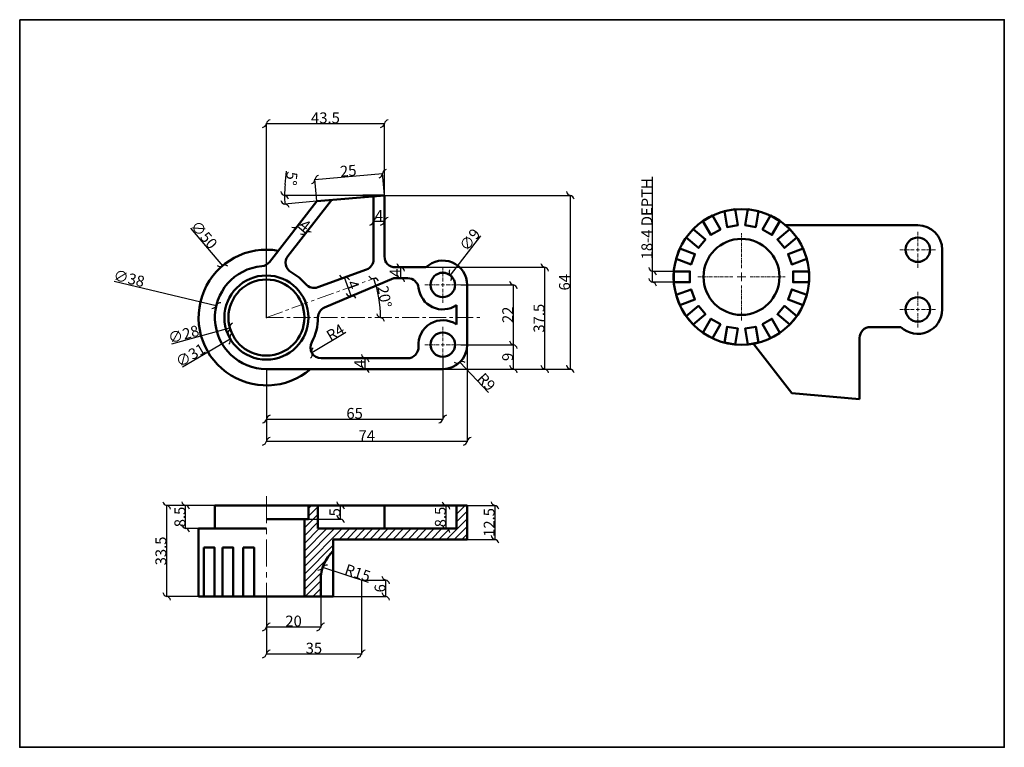
# Model space of a CAD drawing. Units: millimetres. Extents: x 359 to 722, y 83 to 351.
import ezdxf

# ---------------------------------------------------------------- set-up
doc = ezdxf.new("R2010")
doc.units = ezdxf.units.MM
doc.header["$MEASUREMENT"] = 0
doc.linetypes.add('CENTER', pattern=[2, 1.25, -0.25, 0.25, -0.25])
for name, color, linetype, lineweight in [('M-CNTR', 1, 'CENTER', 18), ('M-DIMS', 2, 'Continuous', 25), ('M-HATC', 8, 'Continuous', 18), ('M-OUTL', 7, 'Continuous', 50), ('M-TTLB', 7, 'Continuous', 35)]:
    doc.layers.add(name, color=color, linetype=linetype, lineweight=lineweight)
doc.styles.get("Standard").update_dxf_attribs({"font": 'arial.ttf'})
doc.dimstyles.get("Standard").update_dxf_attribs({"dimtxt": 4, "dimasz": 4, "dimexe": 0.18, "dimexo": 0.0625, "dimgap": 0.09, "dimtad": 1, "dimdec": 0, "dimzin": 0, "dimdsep": 46, "dimtxsty": 'Standard', "dimblk": 'INTEGRAL', "dimcen": 0.09, "dimclre": 251, "dimadec": 0, "dimazin": 0, "dimtfac": 1, "dimtdec": 0, "dimtofl": 0, "dimtmove": 0, "dimatfit": 3, "dimfxl": 1, "dimtolj": 1, "dimtzin": 0, "dimarcsym": 0})

# ---------------------------------------------------------------- blocks, each defined once
blk = doc.blocks.new('*U3')
at = {"layer": 'M-CNTR', "color": 0, "transparency": 16777216}
for p, q in [((0, 1.3), (0, 6.62)), ((-6.62, 0), (-1.3, 0)), ((1.3, 0), (6.62, 0)), ((0, -6.62), (0, -1.3))]:
    blk.add_line(p, q, dxfattribs=at)
at = {"layer": 'M-CNTR', "color": 0, "linetype": 'Continuous', "transparency": 16777216}
for p, q in [((-0.65, 0), (0.65, 0)), ((0, -0.65), (0, 0.65))]:
    blk.add_line(p, q, dxfattribs=at)
blk = doc.blocks.new('*U4')
at = {"layer": 'M-CNTR', "color": 0, "transparency": 16777216}
for p, q in [((0, 1.3), (0, 6.62)), ((-6.62, 0), (-1.3, 0)), ((1.3, 0), (6.62, 0)), ((0, -6.62), (0, -1.3))]:
    blk.add_line(p, q, dxfattribs=at)
at = {"layer": 'M-CNTR', "color": 0, "linetype": 'Continuous', "transparency": 16777216}
for p, q in [((-0.65, 0), (0.65, 0)), ((0, -0.65), (0, 0.65))]:
    blk.add_line(p, q, dxfattribs=at)
blk = doc.blocks.new('*U5')
blk.add_lwpolyline([(-2.96, 2), (2.96, 2), (2.96, -2), (-2.96, -2)], close=True)
blk = doc.blocks.new('*U6')
at = {"layer": 'M-OUTL', "color": 0, "linetype": 'ByBlock', "lineweight": -2, "transparency": 16777216}
for p, rotation in [((736.5, 382.44), 279.9999999999998), ((744.13, 382.44), 259.9999999999998), ((729.34, 379.83), 299.9999999999998), ((751.3, 379.83), 239.9999999999998), ((723.49, 374.93), 319.9999999999998), ((757.14, 374.93), 219.9999999999998), ((719.68, 368.32), 339.9999999999998), ((760.95, 368.32), 199.9999999999998), ((762.28, 360.81), 180), ((719.68, 353.3), 19.99999999999997), ((760.95, 353.3), 159.9999999999998), ((723.49, 346.7), 40), ((757.14, 346.7), 139.9999999999999), ((729.34, 341.79), 59.99999999999992), ((751.3, 341.79), 119.9999999999998), ((736.5, 339.19), 79.99999999999994), ((744.13, 339.19), 99.99999999999989)]:
    blk.add_blockref('*U5', p, dxfattribs=dict(at, rotation=rotation))
blk.add_blockref('*U5', (718.36, 360.81), dxfattribs=at)
blk = doc.blocks.new('*U7')
at = {"layer": 'M-CNTR', "color": 0, "transparency": 16777216}
for p, q in [((0, 3.2), (0, 16.12)), ((-16.12, 0), (-3.2, 0)), ((3.2, 0), (16.12, 0)), ((0, -16.12), (0, -3.2))]:
    blk.add_line(p, q, dxfattribs=at)
at = {"layer": 'M-CNTR', "color": 0, "linetype": 'Continuous', "transparency": 16777216}
for p, q in [((-1.6, 0), (1.6, 0)), ((0, -1.6), (0, 1.6))]:
    blk.add_line(p, q, dxfattribs=at)
blk = doc.blocks.new('*U8')
at = {"layer": 'M-CNTR', "color": 0, "transparency": 16777216}
for p, q in [((0, 1.3), (0, 6.62)), ((-6.62, 0), (-1.3, 0)), ((1.3, 0), (6.62, 0)), ((0, -6.62), (0, -1.3))]:
    blk.add_line(p, q, dxfattribs=at)
at = {"layer": 'M-CNTR', "color": 0, "linetype": 'Continuous', "transparency": 16777216}
for p, q in [((-0.65, 0), (0.65, 0)), ((0, -0.65), (0, 0.65))]:
    blk.add_line(p, q, dxfattribs=at)
blk = doc.blocks.new('*U9')
at = {"layer": 'M-CNTR', "color": 0, "transparency": 16777216}
for p, q in [((0, 1.3), (0, 6.62)), ((-6.62, 0), (-1.3, 0)), ((1.3, 0), (6.62, 0)), ((0, -6.62), (0, -1.3))]:
    blk.add_line(p, q, dxfattribs=at)
at = {"layer": 'M-CNTR', "color": 0, "linetype": 'Continuous', "transparency": 16777216}
for p, q in [((-0.65, 0), (0.65, 0)), ((0, -0.65), (0, 0.65))]:
    blk.add_line(p, q, dxfattribs=at)
blk = doc.blocks.new('_Integral')
at = {"color": 0, "linetype": 'ByBlock', "lineweight": -2}
for centre, start, end in [((0.445, -0.091), 102, 168), ((-0.445, 0.091), 282, 348)]:
    blk.add_arc(centre, 0.454, start, end, dxfattribs=at)
blk = doc.blocks.new('*D10')
at = {"layer": 'Defpoints', "color": 0, "transparency": 16777216}
for p in [(478.48, 256.18), (480.58, 256.94), (483.04, 250.19)]:
    blk.add_point(p, dxfattribs=at)
at = {"layer": 'M-DIMS', "color": 0, "lineweight": -2, "transparency": 16777216}
for p, q in [((480.52, 256.92), (478.31, 256.11)), ((480.93, 249.42), (478.48, 256.18)), ((482.98, 250.17), (480.77, 249.36))]:
    blk.add_line(p, q, dxfattribs=at)
at = {"layer": 'M-DIMS', "color": 0, "lineweight": -2, "transparency": 16777216, "xscale": 4, "yscale": 4, "zscale": 4}
for p, rotation in [((478.48, 256.18), 109.9999999999998), ((480.93, 249.42), 289.9999999999998)]:
    blk.add_blockref('_Integral', p, dxfattribs=dict(at, rotation=rotation))
at = {"layer": 'M-DIMS', "color": 0, "transparency": 16777216, "insert": (481.67, 253.51), "char_height": 4, "attachment_point": 5, "rotation": 290}
blk.add_mtext('\\A1;4', dxfattribs=at)
blk = doc.blocks.new('*D11')
at = {"layer": 'Defpoints', "color": 0, "transparency": 16777216}
for p in [(499.23, 259.95), (499.23, 259.95), (499.23, 255.95)]:
    blk.add_point(p, dxfattribs=at)
at = {"layer": 'M-DIMS', "color": 0, "lineweight": -2, "transparency": 16777216}
for p, q in [((499.23, 255.95), (499.23, 259.95)), ((499.29, 259.95), (499.41, 259.95)), ((499.29, 255.95), (499.41, 255.95))]:
    blk.add_line(p, q, dxfattribs=at)
at = {"layer": 'M-DIMS', "color": 0, "lineweight": -2, "transparency": 16777216, "xscale": 4, "yscale": 4, "zscale": 4}
for p, rotation in [((499.23, 259.95), 90), ((499.23, 255.95), 270)]:
    blk.add_blockref('_Integral', p, dxfattribs=dict(at, rotation=rotation))
at = {"layer": 'M-DIMS', "color": 0, "transparency": 16777216, "insert": (497.14, 257.95), "char_height": 4, "attachment_point": 5, "rotation": 90}
blk.add_mtext('\\A1;4', dxfattribs=at)
blk = doc.blocks.new('*D12')
at = {"layer": 'Defpoints', "color": 0, "transparency": 16777216}
for p in [(489.23, 276.95), (493.23, 276.95), (493.23, 276.95)]:
    blk.add_point(p, dxfattribs=at)
at = {"layer": 'M-DIMS', "color": 0, "lineweight": -2, "transparency": 16777216}
for p, q in [((489.23, 277.01), (489.23, 277.13)), ((489.23, 276.95), (493.23, 276.95)), ((493.23, 277.01), (493.23, 277.13))]:
    blk.add_line(p, q, dxfattribs=at)
at = {"layer": 'M-DIMS', "color": 0, "lineweight": -2, "transparency": 16777216, "xscale": 4, "yscale": 4, "zscale": 4, "rotation": 180}
blk.add_blockref('_Integral', (489.23, 276.95), dxfattribs=at)
at = {"layer": 'M-DIMS', "color": 0, "lineweight": -2, "transparency": 16777216, "xscale": 4, "yscale": 4, "zscale": 4}
blk.add_blockref('_Integral', (493.23, 276.95), dxfattribs=at)
at = {"layer": 'M-DIMS', "color": 0, "transparency": 16777216, "insert": (491.23, 279.04), "char_height": 4, "attachment_point": 5}
blk.add_mtext('\\A1;4', dxfattribs=at)
blk = doc.blocks.new('*D13')
at = {"layer": 'Defpoints', "color": 0, "transparency": 16777216}
for p in [(459.59, 273.09), (464.28, 272.59), (462.74, 270.63)]:
    blk.add_point(p, dxfattribs=at)
at = {"layer": 'M-DIMS', "color": 0, "lineweight": -2, "transparency": 16777216}
for p, q in [((459.63, 273.14), (461.23, 275.19)), ((461.12, 275.05), (464.28, 272.59)), ((462.78, 270.68), (464.39, 272.73))]:
    blk.add_line(p, q, dxfattribs=at)
at = {"layer": 'M-DIMS', "color": 0, "lineweight": -2, "transparency": 16777216, "xscale": 4, "yscale": 4, "zscale": 4}
for p, rotation in [((461.12, 275.05), 142.0238383905026), ((464.28, 272.59), 322.0238383905027)]:
    blk.add_blockref('_Integral', p, dxfattribs=dict(at, rotation=rotation))
at = {"layer": 'M-DIMS', "color": 0, "transparency": 16777216, "insert": (463.98, 275.47), "char_height": 4, "attachment_point": 5, "rotation": 322.0238}
blk.add_mtext('\\A1;4', dxfattribs=at)
blk = doc.blocks.new('*D14')
at = {"layer": 'Defpoints', "color": 0, "transparency": 16777216}
for p in [(492.53, 294.48), (468.32, 284.28), (493.23, 286.45)]:
    blk.add_point(p, dxfattribs=at)
at = {"layer": 'M-DIMS', "color": 0, "lineweight": -2, "transparency": 16777216}
for p, q in [((467.62, 292.3), (492.53, 294.48)), ((493.22, 286.52), (492.51, 294.66)), ((468.32, 284.34), (467.61, 292.48))]:
    blk.add_line(p, q, dxfattribs=at)
at = {"layer": 'M-DIMS', "color": 0, "lineweight": -2, "transparency": 16777216, "xscale": 4, "yscale": 4, "zscale": 4}
for p, rotation in [((492.53, 294.48), 5.000000000000057), ((467.62, 292.3), 185)]:
    blk.add_blockref('_Integral', p, dxfattribs=dict(at, rotation=rotation))
at = {"layer": 'M-DIMS', "color": 0, "transparency": 16777216, "insert": (479.89, 295.51), "char_height": 4, "attachment_point": 5, "rotation": 5}
blk.add_mtext('\\A1;25', dxfattribs=at)
blk = doc.blocks.new('*D15')
at = {"layer": 'Defpoints', "color": 0, "transparency": 16777216}
for p in [(456.46, 284.31), (468.32, 284.28), (485.29, 286.45), (493.23, 286.45), (493.23, 286.45)]:
    blk.add_point(p, dxfattribs=at)
at = {"layer": 'M-DIMS', "color": 0, "lineweight": -2, "transparency": 16777216}
for p, q in [((456.61, 290.45), (457.14, 295.34)), ((485.23, 286.45), (456.21, 286.45)), ((468.26, 284.27), (456.36, 283.23))]:
    blk.add_line(p, q, dxfattribs=at)
for start, end in [(173.7749, 180), (180, 185)]:
    blk.add_arc((493.23, 286.45), 36.83, start, end, dxfattribs=at)
at = {"layer": 'M-DIMS', "color": 0, "lineweight": -2, "transparency": 16777216, "xscale": 4, "yscale": 4, "zscale": 4}
for p, rotation in [((456.39, 286.45), 90.00000000000006), ((456.53, 283.24), 275)]:
    blk.add_blockref('_Integral', p, dxfattribs=dict(at, rotation=rotation))
at = {"layer": 'M-DIMS', "color": 0, "transparency": 16777216, "insert": (458.99, 292.66), "char_height": 4, "attachment_point": 5, "rotation": 263.7749}
blk.add_mtext('\\A1;5°', dxfattribs=at)
blk = doc.blocks.new('*D16')
at = {"layer": 'Defpoints', "color": 0, "transparency": 16777216}
for p in [(493.23, 312.88), (493.23, 286.45), (449.73, 241.45)]:
    blk.add_point(p, dxfattribs=at)
at = {"layer": 'M-DIMS', "color": 0, "lineweight": -2, "transparency": 16777216}
for p, q in [((449.73, 241.52), (449.73, 313.06)), ((449.73, 312.88), (493.23, 312.88)), ((493.23, 286.52), (493.23, 313.06))]:
    blk.add_line(p, q, dxfattribs=at)
at = {"layer": 'M-DIMS', "color": 0, "lineweight": -2, "transparency": 16777216, "xscale": 4, "yscale": 4, "zscale": 4, "rotation": 180}
blk.add_blockref('_Integral', (449.73, 312.88), dxfattribs=at)
at = {"layer": 'M-DIMS', "color": 0, "lineweight": -2, "transparency": 16777216, "xscale": 4, "yscale": 4, "zscale": 4}
blk.add_blockref('_Integral', (493.23, 312.88), dxfattribs=at)
at = {"layer": 'M-DIMS', "color": 0, "transparency": 16777216, "insert": (471.48, 315.02), "char_height": 4, "attachment_point": 5}
blk.add_mtext('\\A1;43.5', dxfattribs=at)
blk = doc.blocks.new('*D17')
at = {"layer": 'Defpoints', "color": 0, "transparency": 16777216}
for p in [(490.14, 256.16), (491.51, 246.34), (449.73, 241.45), (449.73, 241.45), (528.33, 241.45)]:
    blk.add_point(p, dxfattribs=at)
at = {"layer": 'M-DIMS', "color": 0, "lineweight": -2, "transparency": 16777216}
blk.add_arc((449.73, 241.45), 42.07, 360, 20, dxfattribs=at)
at = {"layer": 'M-DIMS', "color": 0, "lineweight": -2, "transparency": 16777216, "xscale": 4, "yscale": 4, "zscale": 4}
for p, rotation in [((489.26, 255.84), 109.9999999999999), ((491.79, 241.45), 269.9999999999999)]:
    blk.add_blockref('_Integral', p, dxfattribs=dict(at, rotation=rotation))
at = {"layer": 'M-DIMS', "color": 0, "transparency": 16777216, "insert": (493.26, 249.13), "char_height": 4, "attachment_point": 5, "rotation": 280}
blk.add_mtext('\\A1;20°', dxfattribs=at)
blk = doc.blocks.new('*D18')
at = {"layer": 'Defpoints', "color": 0, "transparency": 16777216}
for p in [(486.16, 226.45), (486.16, 226.45), (486.16, 222.45)]:
    blk.add_point(p, dxfattribs=at)
at = {"layer": 'M-DIMS', "color": 0, "lineweight": -2, "transparency": 16777216}
for p, q in [((486.16, 222.45), (486.16, 226.45)), ((486.22, 226.45), (486.34, 226.45)), ((486.22, 222.45), (486.34, 222.45))]:
    blk.add_line(p, q, dxfattribs=at)
at = {"layer": 'M-DIMS', "color": 0, "lineweight": -2, "transparency": 16777216, "xscale": 4, "yscale": 4, "zscale": 4}
for p, rotation in [((486.16, 226.45), 90), ((486.16, 222.45), 270)]:
    blk.add_blockref('_Integral', p, dxfattribs=dict(at, rotation=rotation))
at = {"layer": 'M-DIMS', "color": 0, "transparency": 16777216, "insert": (484.07, 224.45), "char_height": 4, "attachment_point": 5, "rotation": 90}
blk.add_mtext('\\A1;4', dxfattribs=at)
blk = doc.blocks.new('*D19')
at = {"layer": 'Defpoints', "color": 0, "transparency": 16777216}
for p in [(514.73, 226.95), (449.73, 222.45), (514.73, 204.02)]:
    blk.add_point(p, dxfattribs=at)
at = {"layer": 'M-DIMS', "color": 0, "lineweight": -2, "transparency": 16777216}
for p, q in [((514.73, 226.89), (514.73, 203.84)), ((449.73, 222.39), (449.73, 203.84)), ((449.73, 204.02), (514.73, 204.02))]:
    blk.add_line(p, q, dxfattribs=at)
at = {"layer": 'M-DIMS', "color": 0, "lineweight": -2, "transparency": 16777216, "xscale": 4, "yscale": 4, "zscale": 4, "rotation": 180}
blk.add_blockref('_Integral', (449.73, 204.02), dxfattribs=at)
at = {"layer": 'M-DIMS', "color": 0, "lineweight": -2, "transparency": 16777216, "xscale": 4, "yscale": 4, "zscale": 4}
blk.add_blockref('_Integral', (514.73, 204.02), dxfattribs=at)
at = {"layer": 'M-DIMS', "color": 0, "transparency": 16777216, "insert": (482.23, 206.16), "char_height": 4, "attachment_point": 5}
blk.add_mtext('\\A1;65', dxfattribs=at)
blk = doc.blocks.new('*D20')
at = {"layer": 'Defpoints', "color": 0, "transparency": 16777216}
for p in [(523.73, 231.45), (449.73, 222.45), (523.73, 195.86)]:
    blk.add_point(p, dxfattribs=at)
at = {"layer": 'M-DIMS', "color": 0, "lineweight": -2, "transparency": 16777216}
for p, q in [((523.73, 231.39), (523.73, 195.68)), ((449.73, 222.39), (449.73, 195.68)), ((449.73, 195.86), (523.73, 195.86))]:
    blk.add_line(p, q, dxfattribs=at)
at = {"layer": 'M-DIMS', "color": 0, "lineweight": -2, "transparency": 16777216, "xscale": 4, "yscale": 4, "zscale": 4, "rotation": 180}
blk.add_blockref('_Integral', (449.73, 195.86), dxfattribs=at)
at = {"layer": 'M-DIMS', "color": 0, "lineweight": -2, "transparency": 16777216, "xscale": 4, "yscale": 4, "zscale": 4}
blk.add_blockref('_Integral', (523.73, 195.86), dxfattribs=at)
at = {"layer": 'M-DIMS', "color": 0, "transparency": 16777216, "insert": (486.73, 197.95), "char_height": 4, "attachment_point": 5}
blk.add_mtext('\\A1;74', dxfattribs=at)
blk = doc.blocks.new('*D21')
at = {"layer": 'Defpoints', "color": 0, "transparency": 16777216}
for p in [(514.73, 231.45), (520.95, 224.95)]:
    blk.add_point(p, dxfattribs=at)
at = {"layer": 'M-DIMS', "color": 0, "lineweight": -2, "transparency": 16777216}
for p, q in [((514.64, 231.45), (514.82, 231.45)), ((514.73, 231.36), (514.73, 231.54)), ((531.55, 213.86), (520.95, 224.95))]:
    blk.add_line(p, q, dxfattribs=at)
at = {"layer": 'M-DIMS', "color": 0, "lineweight": -2, "transparency": 16777216, "xscale": 4, "yscale": 4, "zscale": 4, "rotation": 133.7074136120406}
blk.add_blockref('_Integral', (520.95, 224.95), dxfattribs=at)
at = {"layer": 'M-DIMS', "color": 0, "transparency": 16777216, "insert": (530.8, 217.73), "char_height": 4, "attachment_point": 5, "rotation": 313.7074}
blk.add_mtext('\\A1;R9', dxfattribs=at)
blk = doc.blocks.new('*D22')
at = {"layer": 'Defpoints', "color": 0, "transparency": 16777216}
for p in [(517.47, 257.02), (511.99, 249.89)]:
    blk.add_point(p, dxfattribs=at)
at = {"layer": 'M-DIMS', "color": 0, "lineweight": -2, "transparency": 16777216}
for p, q in [((528.65, 271.58), (517.47, 257.02)), ((514.64, 253.45), (514.82, 253.45)), ((514.73, 253.36), (514.73, 253.54))]:
    blk.add_line(p, q, dxfattribs=at)
at = {"layer": 'M-DIMS', "color": 0, "lineweight": -2, "transparency": 16777216, "xscale": 4, "yscale": 4, "zscale": 4, "rotation": 232.4708864299876}
blk.add_blockref('_Integral', (517.47, 257.02), dxfattribs=at)
at = {"layer": 'M-DIMS', "color": 0, "transparency": 16777216, "insert": (524.69, 270.1), "char_height": 4, "attachment_point": 5, "rotation": 52.4709}
blk.add_mtext('\\A1;∅9', dxfattribs=at)
blk = doc.blocks.new('*D23')
at = {"layer": 'Defpoints', "color": 0, "transparency": 16777216}
for p in [(469.93, 230.45), (466.49, 228.41)]:
    blk.add_point(p, dxfattribs=at)
at = {"layer": 'M-DIMS', "color": 0, "lineweight": -2, "transparency": 16777216}
blk.add_line((479.05, 235.88), (466.49, 228.41), dxfattribs=at)
at = {"layer": 'M-DIMS', "color": 0, "lineweight": -2, "transparency": 16777216, "xscale": 4, "yscale": 4, "zscale": 4, "rotation": 210.7140609288461}
blk.add_blockref('_Integral', (466.49, 228.41), dxfattribs=at)
at = {"layer": 'M-DIMS', "color": 0, "transparency": 16777216, "insert": (475.14, 235.98), "char_height": 4, "attachment_point": 5, "rotation": 30.7141}
blk.add_mtext('\\A1;R4', dxfattribs=at)
blk = doc.blocks.new('*D24')
at = {"layer": 'Defpoints', "color": 0, "transparency": 16777216}
for p in [(433.53, 260.5), (465.92, 222.41)]:
    blk.add_point(p, dxfattribs=at)
at = {"layer": 'M-DIMS', "color": 0, "lineweight": -2, "transparency": 16777216}
for p, q in [((421.71, 274.4), (433.53, 260.5)), ((449.64, 241.45), (449.82, 241.45)), ((449.73, 241.36), (449.73, 241.54))]:
    blk.add_line(p, q, dxfattribs=at)
at = {"layer": 'M-DIMS', "color": 0, "lineweight": -2, "transparency": 16777216, "xscale": 4, "yscale": 4, "zscale": 4, "rotation": 310.3745503375624}
blk.add_blockref('_Integral', (433.53, 260.5), dxfattribs=at)
at = {"layer": 'M-DIMS', "color": 0, "transparency": 16777216, "insert": (426.74, 271.95), "char_height": 4, "attachment_point": 5, "rotation": 310.3746}
blk.add_mtext('\\A1;∅50', dxfattribs=at)
blk = doc.blocks.new('*D25')
at = {"layer": 'Defpoints', "color": 0, "transparency": 16777216}
for p in [(431.25, 245.88), (468.21, 237.03)]:
    blk.add_point(p, dxfattribs=at)
at = {"layer": 'M-DIMS', "color": 0, "lineweight": -2, "transparency": 16777216}
for p, q in [((393.59, 254.91), (431.25, 245.88)), ((449.64, 241.45), (449.82, 241.45)), ((449.73, 241.36), (449.73, 241.54))]:
    blk.add_line(p, q, dxfattribs=at)
at = {"layer": 'M-DIMS', "color": 0, "lineweight": -2, "transparency": 16777216, "xscale": 4, "yscale": 4, "zscale": 4, "rotation": 346.5248169690589}
blk.add_blockref('_Integral', (431.25, 245.88), dxfattribs=at)
at = {"layer": 'M-DIMS', "color": 0, "transparency": 16777216, "insert": (399.11, 255.89), "char_height": 4, "attachment_point": 5, "rotation": 346.5248}
blk.add_mtext('\\A1;∅38', dxfattribs=at)
blk = doc.blocks.new('*D26')
at = {"layer": 'Defpoints', "color": 0, "transparency": 16777216}
for p in [(521.35, 231.45), (540.76, 231.45), (514.73, 222.45)]:
    blk.add_point(p, dxfattribs=at)
at = {"layer": 'M-DIMS', "color": 0, "lineweight": -2, "transparency": 16777216}
for p, q in [((521.41, 231.45), (540.94, 231.45)), ((540.76, 222.45), (540.76, 231.45)), ((514.79, 222.45), (540.94, 222.45))]:
    blk.add_line(p, q, dxfattribs=at)
at = {"layer": 'M-DIMS', "color": 0, "lineweight": -2, "transparency": 16777216, "xscale": 4, "yscale": 4, "zscale": 4}
for p, rotation in [((540.76, 231.45), 90), ((540.76, 222.45), 270)]:
    blk.add_blockref('_Integral', p, dxfattribs=dict(at, rotation=rotation))
at = {"layer": 'M-DIMS', "color": 0, "transparency": 16777216, "insert": (538.63, 226.95), "char_height": 4, "attachment_point": 5, "rotation": 90}
blk.add_mtext('\\A1;9', dxfattribs=at)
blk = doc.blocks.new('*D27')
at = {"layer": 'Defpoints', "color": 0, "transparency": 16777216}
for p in [(521.35, 253.45), (540.76, 253.45), (521.35, 231.45)]:
    blk.add_point(p, dxfattribs=at)
at = {"layer": 'M-DIMS', "color": 0, "lineweight": -2, "transparency": 16777216}
for p, q in [((521.41, 253.45), (540.94, 253.45)), ((540.76, 231.45), (540.76, 253.45)), ((521.41, 231.45), (540.94, 231.45))]:
    blk.add_line(p, q, dxfattribs=at)
at = {"layer": 'M-DIMS', "color": 0, "lineweight": -2, "transparency": 16777216, "xscale": 4, "yscale": 4, "zscale": 4}
for p, rotation in [((540.76, 253.45), 90), ((540.76, 231.45), 270)]:
    blk.add_blockref('_Integral', p, dxfattribs=dict(at, rotation=rotation))
at = {"layer": 'M-DIMS', "color": 0, "transparency": 16777216, "insert": (538.66, 242.45), "char_height": 4, "attachment_point": 5, "rotation": 90}
blk.add_mtext('\\A1;22', dxfattribs=at)
blk = doc.blocks.new('*D28')
at = {"layer": 'Defpoints', "color": 0, "transparency": 16777216}
for p in [(508.5, 259.95), (552.31, 259.95), (514.73, 222.45)]:
    blk.add_point(p, dxfattribs=at)
at = {"layer": 'M-DIMS', "color": 0, "lineweight": -2, "transparency": 16777216}
for p, q in [((508.57, 259.95), (552.49, 259.95)), ((552.31, 222.45), (552.31, 259.95)), ((514.79, 222.45), (552.49, 222.45))]:
    blk.add_line(p, q, dxfattribs=at)
at = {"layer": 'M-DIMS', "color": 0, "lineweight": -2, "transparency": 16777216, "xscale": 4, "yscale": 4, "zscale": 4}
for p, rotation in [((552.31, 259.95), 90), ((552.31, 222.45), 270)]:
    blk.add_blockref('_Integral', p, dxfattribs=dict(at, rotation=rotation))
at = {"layer": 'M-DIMS', "color": 0, "transparency": 16777216, "insert": (550.17, 241.2), "char_height": 4, "attachment_point": 5, "rotation": 90}
blk.add_mtext('\\A1;37.5', dxfattribs=at)
blk = doc.blocks.new('*D29')
at = {"layer": 'Defpoints', "color": 0, "transparency": 16777216}
for p in [(493.23, 286.45), (514.73, 222.45), (561.72, 222.45)]:
    blk.add_point(p, dxfattribs=at)
at = {"layer": 'M-DIMS', "color": 0, "lineweight": -2, "transparency": 16777216}
for p, q in [((493.29, 286.45), (561.9, 286.45)), ((561.72, 286.45), (561.72, 222.45)), ((514.79, 222.45), (561.9, 222.45))]:
    blk.add_line(p, q, dxfattribs=at)
at = {"layer": 'M-DIMS', "color": 0, "lineweight": -2, "transparency": 16777216, "xscale": 4, "yscale": 4, "zscale": 4}
for p, rotation in [((561.72, 286.45), 90), ((561.72, 222.45), 270)]:
    blk.add_blockref('_Integral', p, dxfattribs=dict(at, rotation=rotation))
at = {"layer": 'M-DIMS', "color": 0, "transparency": 16777216, "insert": (559.58, 254.45), "char_height": 4, "attachment_point": 5, "rotation": 90}
blk.add_mtext('\\A1;64', dxfattribs=at)
blk = doc.blocks.new('*D30')
at = {"layer": 'Defpoints', "color": 0, "transparency": 16777216}
for p in [(592.08, 258.43), (599.89, 258.43), (599.89, 254.43)]:
    blk.add_point(p, dxfattribs=at)
at = {"layer": 'M-DIMS', "color": 0, "lineweight": -2, "transparency": 16777216}
for p, q in [((592.08, 258.43), (592.08, 293.23)), ((599.82, 258.43), (591.9, 258.43)), ((592.08, 254.43), (592.08, 258.43)), ((599.82, 254.43), (591.9, 254.43))]:
    blk.add_line(p, q, dxfattribs=at)
at = {"layer": 'M-DIMS', "color": 0, "lineweight": -2, "transparency": 16777216, "xscale": 4, "yscale": 4, "zscale": 4}
for p, rotation in [((592.08, 258.43), 90), ((592.08, 254.43), 270)]:
    blk.add_blockref('_Integral', p, dxfattribs=dict(at, rotation=rotation))
at = {"layer": 'M-DIMS', "color": 0, "transparency": 16777216, "insert": (589.95, 277.83), "char_height": 4, "attachment_point": 5, "rotation": 90}
blk.add_mtext('\\A1;18-4 DEPTH', dxfattribs=at)
blk = doc.blocks.new('*D31')
at = {"layer": 'Defpoints', "color": 0, "transparency": 16777216}
for p in [(412.96, 172.21), (430.73, 172.21), (424.73, 138.71)]:
    blk.add_point(p, dxfattribs=at)
at = {"layer": 'M-DIMS', "color": 0, "lineweight": -2, "transparency": 16777216}
for p, q in [((430.67, 172.21), (412.78, 172.21)), ((412.96, 138.71), (412.96, 172.21)), ((424.67, 138.71), (412.78, 138.71))]:
    blk.add_line(p, q, dxfattribs=at)
at = {"layer": 'M-DIMS', "color": 0, "lineweight": -2, "transparency": 16777216, "xscale": 4, "yscale": 4, "zscale": 4}
for p, rotation in [((412.96, 172.21), 90), ((412.96, 138.71), 270)]:
    blk.add_blockref('_Integral', p, dxfattribs=dict(at, rotation=rotation))
at = {"layer": 'M-DIMS', "color": 0, "transparency": 16777216, "insert": (410.82, 155.46), "char_height": 4, "attachment_point": 5, "rotation": 90}
blk.add_mtext('\\A1;33.5', dxfattribs=at)
blk = doc.blocks.new('*D32')
at = {"layer": 'Defpoints', "color": 0, "transparency": 16777216}
for p in [(419.95, 172.21), (430.73, 172.21), (424.73, 163.75)]:
    blk.add_point(p, dxfattribs=at)
at = {"layer": 'M-DIMS', "color": 0, "lineweight": -2, "transparency": 16777216}
for p, q in [((430.67, 172.21), (419.77, 172.21)), ((419.95, 163.75), (419.95, 172.21)), ((424.67, 163.75), (419.77, 163.75))]:
    blk.add_line(p, q, dxfattribs=at)
at = {"layer": 'M-DIMS', "color": 0, "lineweight": -2, "transparency": 16777216, "xscale": 4, "yscale": 4, "zscale": 4}
for p, rotation in [((419.95, 172.21), 90), ((419.95, 163.75), 270)]:
    blk.add_blockref('_Integral', p, dxfattribs=dict(at, rotation=rotation))
at = {"layer": 'M-DIMS', "color": 0, "transparency": 16777216, "insert": (417.82, 167.98), "char_height": 4, "attachment_point": 5, "rotation": 90}
blk.add_mtext('\\A1;8.5', dxfattribs=at)
blk = doc.blocks.new('*D33')
at = {"layer": 'Defpoints', "color": 0, "transparency": 16777216}
for p in [(463.21, 245.22), (436.24, 237.69)]:
    blk.add_point(p, dxfattribs=at)
at = {"layer": 'M-DIMS', "color": 0, "lineweight": -2, "transparency": 16777216}
for p, q in [((449.64, 241.45), (449.82, 241.45)), ((449.73, 241.36), (449.73, 241.54)), ((414.86, 231.73), (436.24, 237.69))]:
    blk.add_line(p, q, dxfattribs=at)
at = {"layer": 'M-DIMS', "color": 0, "lineweight": -2, "transparency": 16777216, "xscale": 4, "yscale": 4, "zscale": 4, "rotation": 15.58814690371275}
blk.add_blockref('_Integral', (436.24, 237.69), dxfattribs=at)
at = {"layer": 'M-DIMS', "color": 0, "transparency": 16777216, "insert": (419.2, 235.27), "char_height": 4, "attachment_point": 5, "rotation": 15.5881}
blk.add_mtext('\\A1;∅28', dxfattribs=at)
blk = doc.blocks.new('*D34')
at = {"layer": 'Defpoints', "color": 0, "transparency": 16777216}
for p in [(463.08, 249.32), (436.37, 233.59)]:
    blk.add_point(p, dxfattribs=at)
at = {"layer": 'M-DIMS', "color": 0, "lineweight": -2, "transparency": 16777216}
for p, q in [((449.64, 241.45), (449.82, 241.45)), ((449.73, 241.36), (449.73, 241.54)), ((418.8, 223.24), (436.37, 233.59))]:
    blk.add_line(p, q, dxfattribs=at)
at = {"layer": 'M-DIMS', "color": 0, "lineweight": -2, "transparency": 16777216, "xscale": 4, "yscale": 4, "zscale": 4, "rotation": 30.4991865563461}
blk.add_blockref('_Integral', (436.37, 233.59), dxfattribs=at)
at = {"layer": 'M-DIMS', "color": 0, "transparency": 16777216, "insert": (421.75, 227.58), "char_height": 4, "attachment_point": 5, "rotation": 30.4992}
blk.add_mtext('\\A1;∅31', dxfattribs=at)
blk = doc.blocks.new('*D35')
at = {"layer": 'Defpoints', "color": 0, "transparency": 16777216}
for p in [(472.86, 172.21), (477.08, 172.21), (465.23, 167.21)]:
    blk.add_point(p, dxfattribs=at)
at = {"layer": 'M-DIMS', "color": 0, "lineweight": -2, "transparency": 16777216}
for p, q in [((472.92, 172.21), (477.26, 172.21)), ((477.08, 167.21), (477.08, 172.21)), ((465.29, 167.21), (477.26, 167.21))]:
    blk.add_line(p, q, dxfattribs=at)
at = {"layer": 'M-DIMS', "color": 0, "lineweight": -2, "transparency": 16777216, "xscale": 4, "yscale": 4, "zscale": 4}
for p, rotation in [((477.08, 172.21), 90), ((477.08, 167.21), 270)]:
    blk.add_blockref('_Integral', p, dxfattribs=dict(at, rotation=rotation))
at = {"layer": 'M-DIMS', "color": 0, "transparency": 16777216, "insert": (474.95, 169.71), "char_height": 4, "attachment_point": 5, "rotation": 90}
blk.add_mtext('\\A1;5', dxfattribs=at)
blk = doc.blocks.new('*D36')
at = {"layer": 'Defpoints', "color": 0, "transparency": 16777216}
for p in [(515.97, 172.21), (519.73, 172.21), (519.73, 163.71)]:
    blk.add_point(p, dxfattribs=at)
at = {"layer": 'M-DIMS', "color": 0, "lineweight": -2, "transparency": 16777216}
for p, q in [((519.67, 172.21), (515.79, 172.21)), ((515.97, 163.71), (515.97, 172.21)), ((519.67, 163.71), (515.79, 163.71))]:
    blk.add_line(p, q, dxfattribs=at)
at = {"layer": 'M-DIMS', "color": 0, "lineweight": -2, "transparency": 16777216, "xscale": 4, "yscale": 4, "zscale": 4}
for p, rotation in [((515.97, 172.21), 90), ((515.97, 163.71), 270)]:
    blk.add_blockref('_Integral', p, dxfattribs=dict(at, rotation=rotation))
at = {"layer": 'M-DIMS', "color": 0, "transparency": 16777216, "insert": (513.83, 167.96), "char_height": 4, "attachment_point": 5, "rotation": 90}
blk.add_mtext('\\A1;8.5', dxfattribs=at)
blk = doc.blocks.new('*D37')
at = {"layer": 'Defpoints', "color": 0, "transparency": 16777216}
for p in [(523.73, 172.21), (523.73, 159.71), (533.95, 159.71)]:
    blk.add_point(p, dxfattribs=at)
at = {"layer": 'M-DIMS', "color": 0, "lineweight": -2, "transparency": 16777216}
for p, q in [((523.79, 172.21), (534.13, 172.21)), ((533.95, 172.21), (533.95, 159.71)), ((523.79, 159.71), (534.13, 159.71))]:
    blk.add_line(p, q, dxfattribs=at)
at = {"layer": 'M-DIMS', "color": 0, "lineweight": -2, "transparency": 16777216, "xscale": 4, "yscale": 4, "zscale": 4}
for p, rotation in [((533.95, 172.21), 90), ((533.95, 159.71), 270)]:
    blk.add_blockref('_Integral', p, dxfattribs=dict(at, rotation=rotation))
at = {"layer": 'M-DIMS', "color": 0, "transparency": 16777216, "insert": (531.81, 165.96), "char_height": 4, "attachment_point": 5, "rotation": 90}
blk.add_mtext('\\A1;12.5', dxfattribs=at)
blk = doc.blocks.new('*D38')
at = {"layer": 'Defpoints', "color": 0, "transparency": 16777216}
for p in [(469.73, 138.71), (449.73, 134.63), (469.73, 127.5)]:
    blk.add_point(p, dxfattribs=at)
at = {"layer": 'M-DIMS', "color": 0, "lineweight": -2, "transparency": 16777216}
for p, q in [((469.73, 138.65), (469.73, 127.32)), ((449.73, 134.57), (449.73, 127.32)), ((449.73, 127.5), (469.73, 127.5))]:
    blk.add_line(p, q, dxfattribs=at)
at = {"layer": 'M-DIMS', "color": 0, "lineweight": -2, "transparency": 16777216, "xscale": 4, "yscale": 4, "zscale": 4, "rotation": 180}
blk.add_blockref('_Integral', (449.73, 127.5), dxfattribs=at)
at = {"layer": 'M-DIMS', "color": 0, "lineweight": -2, "transparency": 16777216, "xscale": 4, "yscale": 4, "zscale": 4}
blk.add_blockref('_Integral', (469.73, 127.5), dxfattribs=at)
at = {"layer": 'M-DIMS', "color": 0, "transparency": 16777216, "insert": (459.73, 129.63), "char_height": 4, "attachment_point": 5}
blk.add_mtext('\\A1;20', dxfattribs=at)
blk = doc.blocks.new('*D39')
at = {"layer": 'Defpoints', "color": 0, "transparency": 16777216}
for p in [(484.73, 144.71), (449.73, 138.71), (484.73, 117.52)]:
    blk.add_point(p, dxfattribs=at)
at = {"layer": 'M-DIMS', "color": 0, "lineweight": -2, "transparency": 16777216}
for p, q in [((484.73, 144.65), (484.73, 117.34)), ((449.73, 138.65), (449.73, 117.34)), ((449.73, 117.52), (484.73, 117.52))]:
    blk.add_line(p, q, dxfattribs=at)
at = {"layer": 'M-DIMS', "color": 0, "lineweight": -2, "transparency": 16777216, "xscale": 4, "yscale": 4, "zscale": 4, "rotation": 180}
blk.add_blockref('_Integral', (449.73, 117.52), dxfattribs=at)
at = {"layer": 'M-DIMS', "color": 0, "lineweight": -2, "transparency": 16777216, "xscale": 4, "yscale": 4, "zscale": 4}
blk.add_blockref('_Integral', (484.73, 117.52), dxfattribs=at)
at = {"layer": 'M-DIMS', "color": 0, "transparency": 16777216, "insert": (467.23, 119.65), "char_height": 4, "attachment_point": 5}
blk.add_mtext('\\A1;35', dxfattribs=at)
blk = doc.blocks.new('*D40')
at = {"layer": 'Defpoints', "color": 0, "transparency": 16777216}
for p in [(484.73, 144.71), (493.73, 144.71), (474.34, 138.71)]:
    blk.add_point(p, dxfattribs=at)
at = {"layer": 'M-DIMS', "color": 0, "lineweight": -2, "transparency": 16777216}
for p, q in [((484.79, 144.71), (493.91, 144.71)), ((493.73, 138.71), (493.73, 144.71)), ((474.41, 138.71), (493.91, 138.71))]:
    blk.add_line(p, q, dxfattribs=at)
at = {"layer": 'M-DIMS', "color": 0, "lineweight": -2, "transparency": 16777216, "xscale": 4, "yscale": 4, "zscale": 4}
for p, rotation in [((493.73, 144.71), 90), ((493.73, 138.71), 270)]:
    blk.add_blockref('_Integral', p, dxfattribs=dict(at, rotation=rotation))
at = {"layer": 'M-DIMS', "color": 0, "transparency": 16777216, "insert": (491.6, 141.71), "char_height": 4, "attachment_point": 5, "rotation": 90}
blk.add_mtext('\\A1;6', dxfattribs=at)
blk = doc.blocks.new('*D41')
at = {"layer": 'Defpoints', "color": 0, "transparency": 16777216}
for p in [(470.46, 149.34), (484.73, 144.71)]:
    blk.add_point(p, dxfattribs=at)
at = {"layer": 'M-DIMS', "color": 0, "lineweight": -2, "transparency": 16777216}
blk.add_line((487.36, 143.86), (470.46, 149.34), dxfattribs=at)
at = {"layer": 'M-DIMS', "color": 0, "lineweight": -2, "transparency": 16777216, "xscale": 4, "yscale": 4, "zscale": 4, "rotation": 162.0183349135969}
blk.add_blockref('_Integral', (470.46, 149.34), dxfattribs=at)
at = {"layer": 'M-DIMS', "color": 0, "transparency": 16777216, "insert": (483.37, 147.39), "char_height": 4, "attachment_point": 5, "rotation": 342.0183}
blk.add_mtext('\\A1;R15', dxfattribs=at)
blk = doc.blocks.new('FIN-SLOT')
blk.add_lwpolyline([(426.65, 156.71), (430.65, 156.71), (430.65, 138.71), (426.65, 138.71)], close=True)

msp = doc.modelspace()

# ---------------------------------------------------------------- hatches: boundary and pattern name
at = {"layer": 'M-HATC'}
h = msp.add_hatch(dxfattribs=at)
h.set_pattern_fill('ANSI31', color=256, scale=16)
h.paths.add_polyline_path([(463.73, 138.71), (469.73, 138.71), (469.73, 144.71, -0.204278), (474.34, 155.54), (474.34, 159.71), (523.73, 159.71), (523.73, 172.21), (519.73, 172.21), (519.73, 163.71), (468.73, 163.71), (468.73, 172.21), (465.23, 172.21), (465.23, 167.21), (463.73, 167.21)])

# ---------------------------------------------------------------- linework, layer by layer
at = {"layer": 'M-CNTR', "ltscale": 5}
for q in [(490.14, 256.16), (528.33, 241.45)]:
    msp.add_line((449.73, 241.45), q, dxfattribs=at)
at = {"layer": 'M-CNTR', "ltscale": 8}
msp.add_line((449.73, 175.69), (449.73, 134.63), dxfattribs=at)
at = {"layer": 'M-OUTL'}
for p, q in [((468.32, 284.28), (450.86, 261.9)), ((473.77, 284.75), (457.63, 264.08)), ((493.23, 286.45), (468.32, 284.28)), ((493.23, 286.45), (485.29, 286.45)), ((493.23, 286.45), (485.42, 285.77)), ((489.23, 262.89), (489.23, 286.1)), ((493.23, 263.95), (493.23, 286.45)), ((641.05, 275.43), (689.81, 275.43)), ((698.81, 266.43), (698.81, 244.43)), ((468.62, 252.59), (486.6, 259.13)), ((508.5, 259.95), (497.23, 259.95)), ((471.17, 245.16), (496.64, 255.95)), ((501.82, 255.95), (496.64, 255.95)), ((523.73, 231.45), (523.73, 253.45)), ((519.73, 238.94), (519.73, 245.97)), ((683.58, 237.93), (672.31, 237.93)), ((668.31, 233.93), (668.31, 211.43)), ((643.4, 213.61), (629.19, 231.82)), ((501.77, 226.45), (469.93, 226.45)), ((449.73, 222.45), (514.73, 222.45)), ((668.31, 211.43), (643.4, 213.61)), ((430.73, 163.71), (430.73, 172.21)), ((430.73, 172.21), (523.73, 172.21)), ((465.23, 167.21), (465.23, 172.21)), ((468.73, 163.71), (468.73, 172.21)), ((493.23, 172.21), (493.23, 163.71)), ((519.73, 172.21), (519.73, 163.71)), ((523.73, 172.21), (523.73, 159.71)), ((449.73, 167.21), (465.23, 167.21)), ((463.73, 167.21), (463.73, 138.71)), ((424.73, 138.71), (424.73, 163.71)), ((424.73, 163.71), (449.73, 163.71)), ((468.73, 163.71), (519.73, 163.71)), ((474.34, 138.71), (474.34, 159.71)), ((523.73, 159.71), (474.34, 159.71)), ((469.73, 144.71), (469.73, 138.71)), ((449.73, 138.71), (424.73, 138.71)), ((449.73, 138.71), (474.34, 138.71))]:
    msp.add_line(p, q, dxfattribs=at)
for centre, radius in [((624.81, 256.43), 25), ((624.81, 256.43), 14), ((689.81, 266.43), 4.5), ((514.73, 253.45), 4.5), ((449.73, 241.45), 15.5), ((449.73, 241.45), 14), ((689.81, 244.43), 4.5), ((514.73, 231.45), 4.5)]:
    msp.add_circle(centre, radius, dxfattribs=at)
for centre, radius, start, end in [((689.81, 266.43), 9, 0, 90), ((449.73, 241.45), 25, 79.9059, 310.5358), ((447.71, 264.37), 4, 275.0422, 322.0238), ((460.79, 261.62), 4, 142.0238, 241.2593), ((485.23, 262.89), 4, 290, 0), ((497.23, 263.95), 4, 180, 270), ((514.73, 253.45), 9, 0, 133.7617), ((449.73, 241.45), 19, 95.0422, 270), ((449.73, 241.45), 19, 40.3544, 61.2593), ((501.82, 251.95), 4, 6.6258, 90), ((467.26, 256.35), 4, 220.3544, 290), ((514.73, 253.45), 9, 186.6258, 303.749), ((472.73, 241.48), 4, 112.9688, 180.0505), ((689.81, 244.43), 9, 226.2383, 0), ((449.73, 241.45), 19, 331.4281, 0.0505), ((514.73, 231.45), 9, 56.251, 184.4117), ((672.31, 233.93), 4, 90, 180), ((469.93, 230.45), 4, 151.4281, 270), ((501.77, 230.45), 4, 270, 4.4117), ((514.73, 231.45), 9, 270, 0), ((484.73, 144.71), 15, 133.8184, 180)]:
    msp.add_arc(centre, radius, start, end, dxfattribs=at)
at = {"layer": 'M-TTLB'}
msp.add_lwpolyline([(358.79, 351.17), (721.68, 351.17), (721.68, 83.13), (358.79, 83.13)], close=True, dxfattribs=at)

# ---------------------------------------------------------------- block references
at = {"layer": 'M-CNTR'}
for name, p in [('*U7', (624.81, 256.43)), ('*U3', (689.81, 266.43)), ('*U8', (514.73, 253.45)), ('*U4', (689.81, 244.43)), ('*U9', (514.73, 231.45))]:
    msp.add_blockref(name, p, dxfattribs=at)
at = {"layer": 'M-OUTL'}
for name, p in [('*U6', (-115.51, -104.38)), ('FIN-SLOT', (0, 0)), ('FIN-SLOT', (6.84, 0)), ('FIN-SLOT', (14.55, 0))]:
    msp.add_blockref(name, p, dxfattribs=at)

# ---------------------------------------------------------------- dimensions: what is measured, and where the dimension line sits
at = {"layer": 'M-DIMS'}
for base, p1, p2, override, picture, middle in [((493.23, 312.88), (449.73, 241.45), (493.23, 286.45), {"dimdec": 1, "dimclrd": 0, "dimclre": 0, "dimclrt": 0}, '*D16', (471.48, 315.02)), ((493.23, 276.95), (489.23, 276.95), (493.23, 276.95), {"dimclrd": 0, "dimclre": 0, "dimclrt": 0}, '*D12', (491.23, 279.04)), ((523.73, 195.86), (449.73, 222.45), (523.73, 231.45), {"dimclrd": 0, "dimclre": 0, "dimclrt": 0}, '*D20', (486.73, 197.95)), ((514.73, 204.02), (449.73, 222.45), (514.73, 226.95), {"dimclrd": 0, "dimclre": 0, "dimclrt": 0}, '*D19', (482.23, 206.16)), ((484.73, 117.52), (449.73, 138.71), (484.73, 144.71), {"dimclrd": 0, "dimclre": 0, "dimclrt": 0}, '*D39', (467.23, 119.65)), ((469.73, 127.5), (449.73, 134.63), (469.73, 138.71), {"dimclrd": 0, "dimclre": 0, "dimclrt": 0}, '*D38', (459.73, 129.63))]:
    dim = msp.add_linear_dim(base=base, p1=p1, p2=p2, dimstyle='Standard', override=override, dxfattribs=at)
    dim.commit()
    dim.dimension.update_dxf_attribs({"geometry": picture, "text_midpoint": middle})
for p1, p2, distance, picture, middle in [((468.32, 284.28), (493.23, 286.45), 8.05, '*D14', (479.89, 295.51)), ((459.59, 273.09), (462.74, 270.63), 2.49, '*D13', (463.98, 275.47)), ((499.23, 255.95), (499.23, 259.95), 0, '*D11', (497.14, 257.95))]:
    dim = msp.add_aligned_dim(p1=p1, p2=p2, distance=distance, dimstyle='Standard', override={"dimclrd": 0, "dimclre": 0, "dimclrt": 0}, dxfattribs=at)
    dim.commit()
    dim.dimension.update_dxf_attribs({"geometry": picture, "text_midpoint": middle})
for base, line1, line2, picture, middle in [((456.46, 284.31), ((493.23, 286.45), (485.29, 286.45)), ((493.23, 286.45), (468.32, 284.28)), '*D15', (458.99, 292.66)), ((491.51, 246.34), ((449.73, 241.45), (528.33, 241.45)), ((449.73, 241.45), (490.14, 256.16)), '*D17', (493.26, 249.13))]:
    dim = msp.add_angular_dim_2l(base=base, line1=line1, line2=line2, dimstyle='Standard', override={"dimclrd": 0, "dimclre": 0, "dimclrt": 0}, dxfattribs=at)
    dim.commit()
    dim.dimension.update_dxf_attribs({"geometry": picture, "text_midpoint": middle})
dim = msp.add_linear_dim(base=(592.08, 258.43), p1=(599.89, 254.43), p2=(599.89, 258.43), angle=90, text='18-<> DEPTH', dimstyle='Standard', override={"dimclrd": 0, "dimclre": 0, "dimclrt": 0}, dxfattribs=at)
dim.commit()
dim.dimension.update_dxf_attribs({"geometry": '*D30', "text_midpoint": (589.95, 277.83)})
for base, p1, p2, override, picture, middle in [((561.72, 222.45), (493.23, 286.45), (514.73, 222.45), {"dimclrd": 0, "dimclre": 0, "dimclrt": 0}, '*D29', (559.58, 254.45)), ((552.31, 259.95), (514.73, 222.45), (508.5, 259.95), {"dimdec": 1, "dimclrd": 0, "dimclre": 0, "dimclrt": 0}, '*D28', (550.17, 241.2)), ((540.76, 253.45), (521.35, 231.45), (521.35, 253.45), {"dimclrd": 0, "dimclre": 0, "dimclrt": 0, "dimtmove": 1}, '*D27', (538.66, 242.45)), ((540.76, 231.45), (514.73, 222.45), (521.35, 231.45), {"dimclrd": 0, "dimclre": 0, "dimclrt": 0}, '*D26', (538.63, 226.95)), ((486.16, 226.45), (486.16, 222.45), (486.16, 226.45), {"dimclrd": 0, "dimclre": 0, "dimclrt": 0}, '*D18', (484.07, 224.45)), ((412.96, 172.21), (424.73, 138.71), (430.73, 172.21), {"dimdec": 1, "dimclrd": 0, "dimclre": 0, "dimclrt": 0}, '*D31', (410.82, 155.46)), ((419.95, 172.21), (424.73, 163.75), (430.73, 172.21), {"dimdec": 1, "dimclrd": 0, "dimclre": 0, "dimclrt": 0}, '*D32', (417.82, 167.98)), ((477.08, 172.21), (465.23, 167.21), (472.86, 172.21), {"dimclrd": 0, "dimclre": 0, "dimclrt": 0}, '*D35', (474.95, 169.71)), ((515.97, 172.21), (519.73, 163.71), (519.73, 172.21), {"dimdec": 1, "dimclrd": 0, "dimclre": 0, "dimclrt": 0}, '*D36', (513.83, 167.96)), ((533.95, 159.71), (523.73, 172.21), (523.73, 159.71), {"dimdec": 1, "dimclrd": 0, "dimclre": 0, "dimclrt": 0}, '*D37', (531.81, 165.96)), ((493.73, 144.71), (474.34, 138.71), (484.73, 144.71), {"dimclrd": 0, "dimclre": 0, "dimclrt": 0}, '*D40', (491.6, 141.71))]:
    dim = msp.add_linear_dim(base=base, p1=p1, p2=p2, angle=90, dimstyle='Standard', override=override, dxfattribs=at)
    dim.commit()
    dim.dimension.update_dxf_attribs({"geometry": picture, "text_midpoint": middle})
dim = msp.add_diameter_dim_2p(p1=(465.92, 222.41), p2=(433.53, 260.5), dimstyle='Standard', override={"dimclrd": 0, "dimclre": 0, "dimclrt": 0}, dxfattribs=at)
dim.commit()
dim.dimension.update_dxf_attribs({"geometry": '*D24', "text_midpoint": (426.74, 271.95)})
for p1, p2, picture, middle in [((511.99, 249.89), (517.47, 257.02), '*D22', (526.47, 268.74)), ((468.21, 237.03), (431.25, 245.88), '*D25', (398.58, 253.71)), ((463.08, 249.32), (436.37, 233.59), '*D34', (422.89, 225.64)), ((463.21, 245.22), (436.24, 237.69), '*D33', (419.8, 233.11))]:
    dim = msp.add_diameter_dim_2p(p1=p1, p2=p2, dimstyle='Standard', override={"dimclrd": 0, "dimclre": 0, "dimclrt": 0}, dxfattribs=at)
    dim.commit()
    dim.dimension.update_dxf_attribs({"geometry": picture, "text_midpoint": middle, "dimtype": 163})
dim = msp.add_aligned_dim(p1=(483.04, 250.19), p2=(480.58, 256.94), distance=2.24, text='4', dimstyle='Standard', override={"dimclrd": 0, "dimclre": 0, "dimclrt": 0}, dxfattribs=at)
dim.commit()
dim.dimension.update_dxf_attribs({"geometry": '*D10', "text_midpoint": (481.67, 253.51)})
for center, mpoint, picture, middle in [((469.93, 230.45), (466.49, 228.41), '*D23', (476.21, 234.19)), ((514.73, 231.45), (520.95, 224.95), '*D21', (529.26, 216.26)), ((484.73, 144.71), (470.46, 149.34), '*D41', (482.72, 145.37))]:
    dim = msp.add_radius_dim(center=center, mpoint=mpoint, dimstyle='Standard', override={"dimclrd": 0, "dimclre": 0, "dimclrt": 0}, dxfattribs=at)
    dim.commit()
    dim.dimension.update_dxf_attribs({"geometry": picture, "text_midpoint": middle, "dimtype": 164})

doc.saveas('drawing.dxf')
